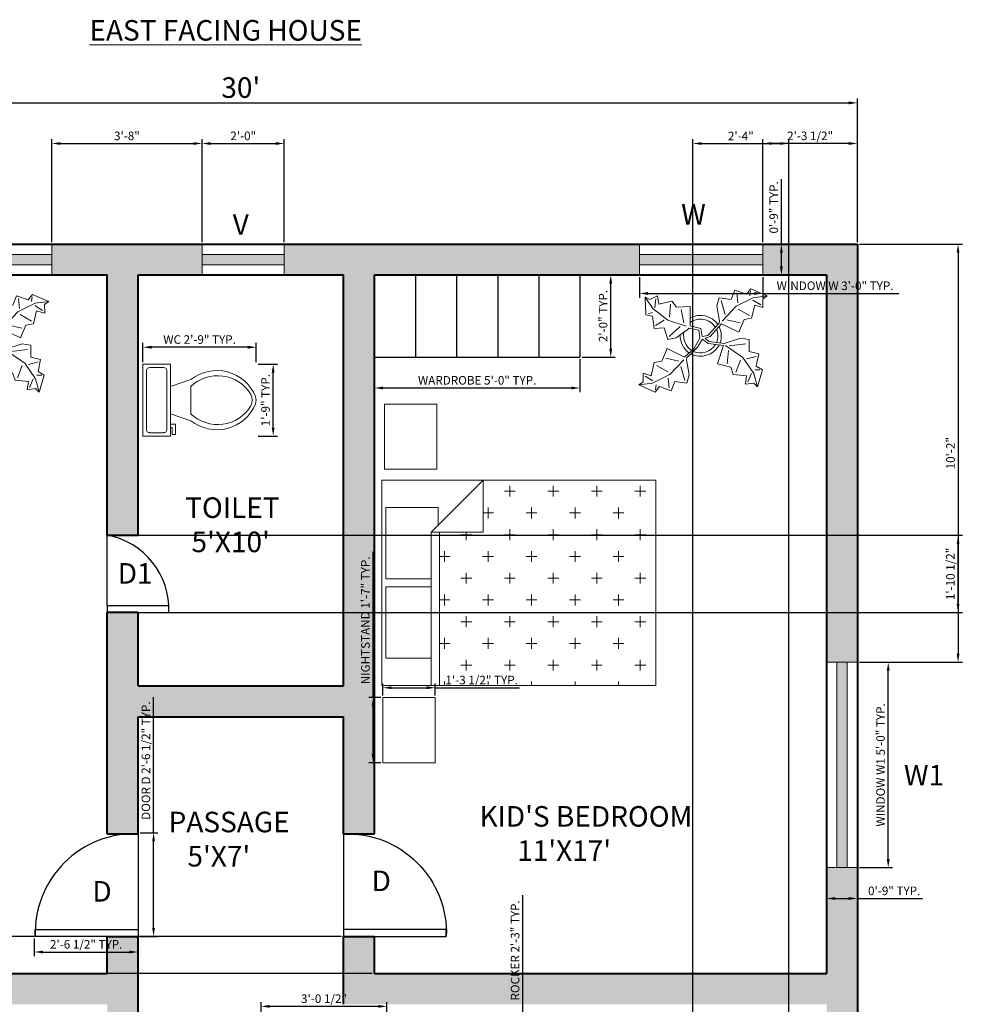
# Model space of a CAD drawing. Units: inches. Extents: x 4432 to 4859, y 8121 to 8698.
# Tile 4 of 4: x 4583 to 4859, y 8410 to 8698. Entities that reach past the tile are written whole.
import ezdxf

# ---------------------------------------------------------------- set-up
doc = ezdxf.new("R2010")
doc.units = ezdxf.units.IN
for name, color, linetype, lineweight in [('A-ANNO-DIMS', 2, 'Continuous', 18), ('A-ANNO-TEXT', 7, 'Continuous', 18), ('A-AREA-IDEN', 4, 'Continuous', 18), ('A-DOOR', 3, 'Continuous', 25), ('A-FLOR-CASE', 8, 'Continuous', 25), ('A-FLOR-FIXT', 9, 'Continuous', 18), ('A-FURN', 8, 'Continuous', 18), ('A-FURN-PATT', 8, 'Continuous', 13), ('A-FURN-PLNT', 94, 'Continuous', 13), ('A-GLAZ', 4, 'Continuous', 20), ('A-GLAZ-PATT', 4, 'Continuous', 13), ('A-WALL', 7, 'Continuous', 40)]:
    doc.layers.add(name, color=color, linetype=linetype, lineweight=lineweight)
doc.layers.add('A-WALL-PATT', color=219, linetype='Continuous', lineweight=13, true_color=0x642165)
doc.styles.get("Standard").update_dxf_attribs({"font": 'arial.ttf'})
doc.dimstyles.new('ISO-25', dxfattribs={"dimtxt": 2.5, "dimasz": 2.5, "dimexe": 1.25, "dimexo": 0.625, "dimtad": 1, "dimlunit": 3, "dimtxsty": 'Standard', "dimcen": 2.5, "dimadec": 0, "dimazin": 0, "dimtfac": 1, "dimtmove": 0, "dimatfit": 3, "dimfxl": 1, "dimarcsym": 0})

# ---------------------------------------------------------------- blocks, each defined once
blk = doc.blocks.new('Bed - Queen')
for p, q in [((0, -80.00003), (0, 0)), ((0, 0), (59.99999, 0)), ((59.99999, 0), (59.99999, -80.00003)), ((7.99999, -1.2), (28.79998, -1.2)), ((7.99999, -14.4), (7.99999, -1.2)), ((28.79998, -1.2), (28.79998, -14.4)), ((31.19999, -1.2), (51.99999, -1.2)), ((31.19999, -14.4), (31.19999, -1.2)), ((51.99999, -1.2), (51.99999, -16.4)), ((0, -14.4), (44.8, -14.4)), ((44.8, -16.8), (0, -16.8)), ((59.99999, -29.6), (44.8, -14.4)), ((44.8, -14.4), (44.8, -29.6)), ((51.99999, -16.4), (46.79936, -16.4)), ((44.8, -29.6), (59.99999, -29.6)), ((59.99999, -80.00003), (0, -80.00003))]:
    blk.add_line(p, q)
blk = doc.blocks.new('Plant - Rubber or Philodendron')
for p, q in [((-14.8639, 10.7964), (-12.6195, 11.8975)), ((-12.6195, 11.8975), (-12.1909, 9.4345)), ((8.8871, 10.7908), (9.9809, 13.4933)), ((9.9809, 13.4933), (13.3837, 12.301)), ((10.5828, 12.6946), (10.8893, 9.7953)), ((13.3837, 12.301), (14.68, 13.9039)), ((14.5816, 13.2037), (14.3848, 11.8033)), ((14.68, 13.9039), (19.3848, 11.8146)), ((19.3848, 11.8146), (15.3859, 11.3055)), ((19.3848, 11.8146), (18.1868, 10.9119)), ((-16.2005, 11.4774), (-13.9899, 8.1064)), ((-16.2005, 11.4774), (-14.8639, 10.7964)), ((-16.0159, 6.3329), (-16.2005, 11.4774)), ((-13.3174, 8.325), (-13.0735, 11.0065)), ((-12.1909, 9.4345), (-8.3829, 10.3)), ((-8.8369, 9.409), (-9.0894, 5.6095)), ((-8.3829, 10.3), (-7.0549, 8.501)), ((-7.0549, 8.501), (-3.0284, 8.6941)), ((-3.0284, 8.6941), (-3.0709, 3.1041)), ((4.6914, 8.8812), (5.3859, 11.2828)), ((4.6914, 8.8812), (5.5014, 4.4831)), ((5.3859, 11.2828), (8.8871, 10.7908)), ((5.9878, 10.4842), (7.1971, 6.3869)), ((10.3916, 8.7942), (6.2847, 4.4028)), ((15.3859, 11.3055), (10.3916, 8.7942)), ((15.7909, 9.1065), (14.8995, 5.3044)), ((15.2875, 10.6053), (17.5907, 9.2105)), ((18.1925, 8.4119), (15.7909, 9.1065)), ((18.1868, 10.9119), (18.1925, 8.4119)), ((-14.0069, 5.8704), (-16.0159, 6.3329)), ((-15.3434, 6.5514), (-13.9984, 6.9884)), ((-13.5868, 2.2894), (-14.0069, 5.8704)), ((-13.9899, 8.1064), (-9.5434, 4.7185)), ((-4.8529, 4.012), (-5.7184, 7.82)), ((14.2977, 6.1031), (10.9934, 7.9956)), ((-13.1329, 3.1804), (-10.6614, 4.727)), ((-9.5434, 4.7185), (-4.1917, 2.9888)), ((-9.1318, 0.0195), (-5.9793, 2.9025)), ((-3.0709, 3.1041), (0.0797, 2.3163)), ((2.1141, 0.2298), (5.4346, 3.9146)), ((6.1032, 3.6844), (2.8262, -0.031)), ((5.4346, 3.9146), (5.5014, 4.4831)), ((11.1089, 1.1958), (6.1032, 3.6844)), ((7.7005, 4.8881), (11.5025, 3.9967)), ((12.7005, 4.8994), (11.1089, 1.1958)), ((14.8995, 5.3044), (12.7005, 4.8994)), ((-10.6784, 2.491), (-13.5868, 2.2894)), ((-9.5858, -0.8715), (-10.6784, 2.491)), ((-7.1228, -0.443), (-3.5248, 2.2131)), ((-3.5248, 2.2131), (-3.3011, 2.4355)), ((-3.3011, 2.4355), (-0.5306, 1.7947)), ((-0.5306, 1.7947), (-0.2255, -0.5527)), ((-0.5306, 1.7947), (-0.5306, 1.7947)), ((0.0797, 2.3163), (0.4866, -0.031)), ((0.4866, -0.031), (2.1141, 0.2298)), ((-7.1228, -0.443), (-9.5858, -0.8715)), ((-2.019, -3.6148), (-0.2255, -0.5527)), ((-0.9375, -3.1608), (0.5883, -0.8135)), ((0.5883, -0.8135), (2.2447, -2.0916)), ((2.8262, -0.031), (1.3003, -0.5527)), ((1.3003, -0.5527), (2.4193, -1.4655)), ((2.2447, -2.0916), (6.7108, -2.6626)), ((2.4193, -1.4655), (6.895, -2.1175)), ((4.943, -7.9659), (6.7108, -2.6626)), ((11.6605, -0.5413), (6.895, -2.1175)), ((12.3677, -6.1981), (7.219, -2.6772)), ((8.3544, -2.7453), (13.1973, -2.1704)), ((11.6605, -0.5413), (14.1354, -0.8948)), ((14.1354, -0.8948), (14.1354, -4.4304)), ((-11.3237, -7.2629), (-9.7321, -3.5593)), ((-9.7321, -3.5593), (-4.7264, -6.0479)), ((-2.019, -3.6148), (-4.7264, -6.0479)), ((-4.0579, -6.2781), (-0.9375, -3.1608)), ((8.125, -4.0768), (7.7715, -7.9659)), ((14.1354, -4.4304), (16.9638, -5.1375)), ((16.9638, -5.1375), (16.2567, -8.673)), ((-14.4141, -11.4699), (-13.5228, -7.6679)), ((-13.5228, -7.6679), (-11.3237, -7.2629)), ((-12.921, -8.4665), (-9.6166, -10.359)), ((-6.3237, -7.2516), (-10.1257, -6.3602)), ((-9.0148, -11.1577), (-4.9047, -6.8122)), ((-4.1246, -6.8466), (-4.0579, -6.2781)), ((-3.3146, -11.2447), (-4.1246, -6.8466)), ((8.8321, -9.0266), (4.943, -7.9659)), ((10.2463, -10.4408), (11.6605, -6.9053)), ((15.5496, -10.7943), (12.3677, -6.1981)), ((16.2567, -5.8446), (13.4283, -6.5517)), ((-16.8157, -10.7754), (-14.4141, -11.4699)), ((-16.8101, -13.2754), (-16.8157, -10.7754)), ((-14.0091, -13.669), (-9.0148, -11.1577)), ((-4.611, -12.8477), (-5.8203, -8.7504)), ((-3.3146, -11.2447), (-4.0092, -13.6463)), ((9.5392, -11.1479), (8.8321, -9.0266)), ((13.4283, -11.5015), (9.5392, -11.1479)), ((13.0748, -13.9763), (13.4283, -11.5015)), ((14.8425, -10.7943), (13.7819, -13.2692)), ((16.6103, -14.6834), (15.5496, -10.7943)), ((17.3174, -9.7337), (15.9032, -9.7337)), ((16.2567, -8.673), (18.0245, -9.7337)), ((18.0245, -9.7337), (16.6103, -14.6834)), ((-18.008, -14.1781), (-16.8101, -13.2754)), ((-18.008, -14.1781), (-14.0091, -13.669)), ((-13.3032, -16.2674), (-18.008, -14.1781)), ((-13.9107, -12.9688), (-16.2139, -11.574)), ((-13.2048, -15.5672), (-13.008, -14.1668)), ((-9.206, -15.0581), (-9.5126, -12.1588)), ((-7.5103, -13.1543), (-8.6042, -15.8568)), ((-4.0092, -13.6463), (-7.5103, -13.1543)), ((15.5496, -13.6228), (13.0748, -13.9763)), ((16.6103, -14.6834), (15.5496, -13.6228)), ((-12.0069, -14.6645), (-13.3032, -16.2674)), ((-8.6042, -15.8568), (-12.0069, -14.6645))]:
    blk.add_line(p, q)
for centre, radius, start, end in [((0, 0), 6.1275, 34.37569, 120.1028), ((-0.0601, -0.2075), 5.2461, 33.82192, 124.9414), ((0.0308, 0.1664), 6, 178.6147, 235.1169), ((0.0308, 0.1664), 5, 168.1647, 238.6725), ((-0.2664, 0.1682), 5.2775, 338.4094, 20.03007), ((-0.098, 0.1364), 6.1288, 341.2017, 26.09184), ((-0.0234, 0.3825), 6.1492, 242.5812, 331.2714), ((-0.1102, 0.4886), 5.2883, 247.3711, 327.472)]:
    blk.add_arc(centre, radius, start, end)
blk = doc.blocks.new('Toilet - top')
for p, q in [((9.5, -6), (9.5, -2)), ((-10, -8.5), (-8, -8.5)), ((-10, -9.5), (-10, -8.5)), ((-8, -8.5), (-8, -8)), ((-7, -8), (-7, -9.5)), ((-4, -8), (-6, -14)), ((4, -8), (6, -14)), ((-7, -9.5), (-10, -9.5)), ((4, -14), (-4, -14))]:
    blk.add_line(p, q)
blk.add_lwpolyline([(10.5, -8), (10.5, 0), (-10.5, 0), (-10.5, -8)], close=True)
for points in [[(-9.5, -2), (-9.5, -6)], [(8.5, -1), (-8.5, -1)], [(-8.5, -7), (8.5, -7)]]:
    blk.add_lwpolyline(points)
for centre, radius, start, end in [((-8.62, -1.88), 0.884, 81.8699, 188.1301), ((8.62, -1.88), 0.884, 351.8699, 98.1301), ((-8.62, -6.12), 0.884, 171.8699, 278.1301), ((8.62, -6.12), 0.884, 261.8699, 8.1301), ((3.52, -21.58), 12.17, 141.4691, 247.9714), ((4.2, -21.82), 11.33, 136.3677, 238.9468), ((-3.52, -21.58), 12.17, 292.0284, 38.5307), ((-4.2, -21.82), 11.33, 301.053, 43.6321), ((0, -27.88), 4, 245.7318, 294.2682), ((0, -29), 4, 254.8605, 285.1395)]:
    blk.add_arc(centre, radius, start, end)
blk = doc.blocks.new('*D14')
at = {"layer": 'A-ANNO-DIMS', "color": 0, "lineweight": -2, "transparency": 16777216}
for p, q in [((4467.47, 8632.58), (4467.47, 8674.47)), ((4469.97, 8673.22), (4824.97, 8673.22)), ((4827.47, 8632.58), (4827.47, 8674.47))]:
    blk.add_line(p, q, dxfattribs=at)
at = {"layer": 'A-ANNO-DIMS', "color": 0, "transparency": 16777216}
for points in [[(4469.97, 8673.64), (4469.97, 8672.8), (4467.47, 8673.22)], [(4824.97, 8673.64), (4824.97, 8672.8), (4827.47, 8673.22)]]:
    blk.add_solid(points, dxfattribs=at)
at = {"layer": 'Defpoints', "color": 0, "transparency": 16777216}
for p in [(4827.47, 8673.22), (4467.47, 8631.96), (4827.47, 8631.96)]:
    blk.add_point(p, dxfattribs=at)
at = {"layer": 'A-ANNO-DIMS', "color": 0, "transparency": 16777216, "insert": (4647.47, 8676.91), "char_height": 6, "attachment_point": 5}
blk.add_mtext("30'", dxfattribs=at)
blk = doc.blocks.new('WIN-36IN')
for p, q in [((0, 0), (0, 9)), ((0, 9), (36, 9)), ((36, 9), (36, 0)), ((0, 6), (36, 6)), ((0, 3), (36, 3)), ((36, 0), (0, 0))]:
    blk.add_line(p, q)
blk = doc.blocks.new('WIN-60IN')
for p, q in [((0, 60), (9, 60)), ((0, 60), (0, 0)), ((3, 60), (3, 0)), ((6, 60), (6, 0)), ((9, 0), (9, 60)), ((0, 0), (9, 0)), ((0, 0), (9, 0))]:
    blk.add_line(p, q)
blk = doc.blocks.new('DOOR-SWING-30IN')
for p, q in [((0, 30), (0, 0)), ((-30, 0), (-30, 2)), ((-30, 2), (0, 2)), ((0, 0), (-30, 0))]:
    blk.add_line(p, q)
blk.add_arc((-1, 1), 29.02, 88.0251, 181.9749)
blk = doc.blocks.new('WARDROBE-5BAY-60IN')
for p, q in [((12, 24), (12, 0)), ((24, 24), (24, 0)), ((36, 24), (36, 0)), ((48, 24), (48, 0)), ((60, 24), (60, 0)), ((0, 0), (60, 0))]:
    blk.add_line(p, q)
blk = doc.blocks.new('NIGHTSTAND-RECT')
blk.add_lwpolyline([(0, 19.04), (15.29, 19.04), (15.29, 0), (0, 0)], close=True)
blk = doc.blocks.new('*D23')
at = {"layer": 'A-ANNO-DIMS', "color": 0, "lineweight": -2, "transparency": 16777216}
for p, q in [((4763.88, 8622.33), (4763.88, 8616.31)), ((4799.88, 8622.33), (4799.88, 8616.31)), ((4766.38, 8617.56), (4797.38, 8617.56)), ((4799.88, 8617.56), (4839.53, 8617.56))]:
    blk.add_line(p, q, dxfattribs=at)
at = {"layer": 'A-ANNO-DIMS', "color": 0, "transparency": 16777216}
for points in [[(4766.38, 8617.97), (4766.38, 8617.14), (4763.88, 8617.56)], [(4797.38, 8617.97), (4797.38, 8617.14), (4799.88, 8617.56)]]:
    blk.add_solid(points, dxfattribs=at)
at = {"layer": 'Defpoints', "color": 0, "transparency": 16777216}
for p in [(4763.88, 8622.96), (4799.88, 8622.96), (4799.88, 8617.56)]:
    blk.add_point(p, dxfattribs=at)
at = {"layer": 'A-ANNO-DIMS', "color": 0, "transparency": 16777216, "insert": (4820.95, 8619.48), "char_height": 2.5, "attachment_point": 5}
blk.add_mtext('WINDOW W 3\'-0" TYP.', dxfattribs=at)
blk = doc.blocks.new('*D24')
at = {"layer": 'A-ANNO-DIMS', "color": 0, "lineweight": -2, "transparency": 16777216}
for p, q in [((4805.28, 8631.96), (4805.28, 8650.95)), ((4800.5, 8631.96), (4806.53, 8631.96)), ((4805.28, 8625.46), (4805.28, 8629.46)), ((4800.5, 8622.96), (4806.53, 8622.96))]:
    blk.add_line(p, q, dxfattribs=at)
at = {"layer": 'A-ANNO-DIMS', "color": 0, "transparency": 16777216}
for points in [[(4804.86, 8629.46), (4805.69, 8629.46), (4805.28, 8631.96)], [(4804.86, 8625.46), (4805.69, 8625.46), (4805.28, 8622.96)]]:
    blk.add_solid(points, dxfattribs=at)
at = {"layer": 'Defpoints', "color": 0, "transparency": 16777216}
for p in [(4799.88, 8631.96), (4805.28, 8631.96), (4799.88, 8622.96)]:
    blk.add_point(p, dxfattribs=at)
at = {"layer": 'A-ANNO-DIMS', "color": 0, "transparency": 16777216, "insert": (4803.38, 8642.7), "char_height": 2.5, "attachment_point": 5, "rotation": 90}
blk.add_mtext('0\'-9" TYP.', dxfattribs=at)
blk = doc.blocks.new('*D25')
at = {"layer": 'A-ANNO-DIMS', "color": 0, "lineweight": -2, "transparency": 16777216}
for p, q in [((4828.09, 8509.87), (4837.72, 8509.87)), ((4836.47, 8452.37), (4836.47, 8507.37)), ((4828.09, 8449.87), (4837.72, 8449.87))]:
    blk.add_line(p, q, dxfattribs=at)
at = {"layer": 'A-ANNO-DIMS', "color": 0, "transparency": 16777216}
for points in [[(4836.05, 8507.37), (4836.88, 8507.37), (4836.47, 8509.87)], [(4836.05, 8452.37), (4836.88, 8452.37), (4836.47, 8449.87)]]:
    blk.add_solid(points, dxfattribs=at)
at = {"layer": 'Defpoints', "color": 0, "transparency": 16777216}
for p in [(4827.47, 8509.87), (4836.47, 8509.87), (4827.47, 8449.87)]:
    blk.add_point(p, dxfattribs=at)
at = {"layer": 'A-ANNO-DIMS', "color": 0, "transparency": 16777216, "insert": (4834.55, 8479.87), "char_height": 2.5, "attachment_point": 5, "rotation": 90}
blk.add_mtext('WINDOW W1 5\'-0" TYP.', dxfattribs=at)
blk = doc.blocks.new('*D26')
at = {"layer": 'A-ANNO-DIMS', "color": 0, "lineweight": -2, "transparency": 16777216}
for p, q in [((4818.47, 8449.25), (4818.47, 8439.62)), ((4827.47, 8449.25), (4827.47, 8439.62)), ((4820.97, 8440.87), (4824.97, 8440.87)), ((4827.47, 8440.87), (4846.46, 8440.87))]:
    blk.add_line(p, q, dxfattribs=at)
at = {"layer": 'A-ANNO-DIMS', "color": 0, "transparency": 16777216}
for points in [[(4820.97, 8441.29), (4820.97, 8440.45), (4818.47, 8440.87)], [(4824.97, 8441.29), (4824.97, 8440.45), (4827.47, 8440.87)]]:
    blk.add_solid(points, dxfattribs=at)
at = {"layer": 'Defpoints', "color": 0, "transparency": 16777216}
for p in [(4818.47, 8449.87), (4827.47, 8449.87), (4827.47, 8440.87)]:
    blk.add_point(p, dxfattribs=at)
at = {"layer": 'A-ANNO-DIMS', "color": 0, "transparency": 16777216, "insert": (4838.21, 8442.77), "char_height": 2.5, "attachment_point": 5}
blk.add_mtext('0\'-9" TYP.', dxfattribs=at)
blk = doc.blocks.new('*D29')
at = {"layer": 'A-ANNO-DIMS', "color": 0, "lineweight": -2, "transparency": 16777216}
for p, q in [((4686.1, 8499.56), (4686.1, 8542.1)), ((4688.33, 8499.56), (4684.85, 8499.56)), ((4686.1, 8483.02), (4686.1, 8497.06)), ((4688.33, 8480.52), (4684.85, 8480.52))]:
    blk.add_line(p, q, dxfattribs=at)
at = {"layer": 'A-ANNO-DIMS', "color": 0, "transparency": 16777216}
for points in [[(4685.68, 8497.06), (4686.51, 8497.06), (4686.1, 8499.56)], [(4685.68, 8483.02), (4686.51, 8483.02), (4686.1, 8480.52)]]:
    blk.add_solid(points, dxfattribs=at)
at = {"layer": 'Defpoints', "color": 0, "transparency": 16777216}
for p in [(4686.1, 8499.56), (4688.95, 8499.56), (4688.95, 8480.52)]:
    blk.add_point(p, dxfattribs=at)
at = {"layer": 'A-ANNO-DIMS', "color": 0, "transparency": 16777216, "insert": (4684.18, 8522.08), "char_height": 2.5, "attachment_point": 5, "rotation": 90}
blk.add_mtext('NIGHTSTAND 1\'-7" TYP.', dxfattribs=at)
blk = doc.blocks.new('*D30')
at = {"layer": 'A-ANNO-DIMS', "color": 0, "lineweight": -2, "transparency": 16777216}
for p, q in [((4688.95, 8500.18), (4688.95, 8503.66)), ((4704.24, 8500.18), (4704.24, 8503.66)), ((4691.45, 8502.41), (4701.74, 8502.41)), ((4704.24, 8502.41), (4728.82, 8502.41))]:
    blk.add_line(p, q, dxfattribs=at)
at = {"layer": 'A-ANNO-DIMS', "color": 0, "transparency": 16777216}
for points in [[(4691.45, 8502.83), (4691.45, 8502), (4688.95, 8502.41)], [(4701.74, 8502.83), (4701.74, 8502), (4704.24, 8502.41)]]:
    blk.add_solid(points, dxfattribs=at)
at = {"layer": 'Defpoints', "color": 0, "transparency": 16777216}
for p in [(4704.24, 8502.41), (4688.95, 8499.56), (4704.24, 8499.56)]:
    blk.add_point(p, dxfattribs=at)
at = {"layer": 'A-ANNO-DIMS', "color": 0, "transparency": 16777216, "insert": (4717.78, 8504.33), "char_height": 2.5, "attachment_point": 5}
blk.add_mtext('1\'-3 1/2" TYP.', dxfattribs=at)
blk = doc.blocks.new('*D31')
at = {"layer": 'A-ANNO-DIMS', "color": 0, "lineweight": -2, "transparency": 16777216}
for p, q in [((4622.01, 8460.05), (4622.01, 8499.68)), ((4618.09, 8460.05), (4623.26, 8460.05)), ((4622.01, 8432.28), (4622.01, 8457.55)), ((4618.09, 8429.78), (4623.26, 8429.78))]:
    blk.add_line(p, q, dxfattribs=at)
at = {"layer": 'A-ANNO-DIMS', "color": 0, "transparency": 16777216}
for points in [[(4621.59, 8457.55), (4622.43, 8457.55), (4622.01, 8460.05)], [(4621.59, 8432.28), (4622.43, 8432.28), (4622.01, 8429.78)]]:
    blk.add_solid(points, dxfattribs=at)
at = {"layer": 'Defpoints', "color": 0, "transparency": 16777216}
for p in [(4617.47, 8460.05), (4622.01, 8460.05), (4617.47, 8429.78)]:
    blk.add_point(p, dxfattribs=at)
at = {"layer": 'A-ANNO-DIMS', "color": 0, "transparency": 16777216, "insert": (4620.09, 8481.12), "char_height": 2.5, "attachment_point": 5, "rotation": 90}
blk.add_mtext('DOOR D 2\'-6 1/2" TYP.', dxfattribs=at)
blk = doc.blocks.new('*D32')
at = {"layer": 'A-ANNO-DIMS', "color": 0, "lineweight": -2, "transparency": 16777216}
for p, q in [((4587.19, 8429.15), (4587.19, 8423.98)), ((4617.47, 8429.15), (4617.47, 8423.98)), ((4589.69, 8425.23), (4614.97, 8425.23))]:
    blk.add_line(p, q, dxfattribs=at)
at = {"layer": 'A-ANNO-DIMS', "color": 0, "transparency": 16777216}
for points in [[(4589.69, 8425.65), (4589.69, 8424.82), (4587.19, 8425.23)], [(4614.97, 8425.65), (4614.97, 8424.82), (4617.47, 8425.23)]]:
    blk.add_solid(points, dxfattribs=at)
at = {"layer": 'Defpoints', "color": 0, "transparency": 16777216}
for p in [(4587.19, 8429.78), (4617.47, 8429.78), (4617.47, 8425.23)]:
    blk.add_point(p, dxfattribs=at)
at = {"layer": 'A-ANNO-DIMS', "color": 0, "transparency": 16777216, "insert": (4602.33, 8427.15), "char_height": 2.5, "attachment_point": 5}
blk.add_mtext('2\'-6 1/2" TYP.', dxfattribs=at)
blk = doc.blocks.new('*D33')
at = {"layer": 'A-ANNO-DIMS', "color": 0, "lineweight": -2, "transparency": 16777216}
for p, q in [((4729.79, 8407.06), (4729.79, 8441.83)), ((4726.37, 8407.06), (4731.04, 8407.06)), ((4729.79, 8382.56), (4729.79, 8404.56)), ((4726.37, 8380.06), (4731.04, 8380.06))]:
    blk.add_line(p, q, dxfattribs=at)
at = {"layer": 'A-ANNO-DIMS', "color": 0, "transparency": 16777216}
for points in [[(4729.38, 8404.56), (4730.21, 8404.56), (4729.79, 8407.06)], [(4729.38, 8382.56), (4730.21, 8382.56), (4729.79, 8380.06)]]:
    blk.add_solid(points, dxfattribs=at)
at = {"layer": 'Defpoints', "color": 0, "transparency": 16777216}
for p in [(4725.74, 8407.06), (4729.79, 8407.06), (4725.74, 8380.06)]:
    blk.add_point(p, dxfattribs=at)
at = {"layer": 'A-ANNO-DIMS', "color": 0, "transparency": 16777216, "insert": (4727.87, 8425.7), "char_height": 2.5, "attachment_point": 5, "rotation": 90}
blk.add_mtext('ROCKER 2\'-3" TYP.', dxfattribs=at)
blk = doc.blocks.new('*D37')
at = {"layer": 'A-ANNO-DIMS', "color": 0, "lineweight": -2, "transparency": 16777216}
for p, q in [((4618.91, 8597.53), (4618.91, 8603.11)), ((4649.46, 8601.86), (4621.41, 8601.86)), ((4651.96, 8597.53), (4651.96, 8603.11))]:
    blk.add_line(p, q, dxfattribs=at)
at = {"layer": 'A-ANNO-DIMS', "color": 0, "transparency": 16777216}
for points in [[(4621.41, 8602.28), (4621.41, 8601.44), (4618.91, 8601.86)], [(4649.46, 8602.28), (4649.46, 8601.44), (4651.96, 8601.86)]]:
    blk.add_solid(points, dxfattribs=at)
at = {"layer": 'Defpoints', "color": 0, "transparency": 16777216}
for p in [(4618.91, 8601.86), (4618.91, 8596.9), (4651.96, 8596.9)]:
    blk.add_point(p, dxfattribs=at)
at = {"layer": 'A-ANNO-DIMS', "color": 0, "transparency": 16777216, "insert": (4635.44, 8603.78), "char_height": 2.5, "attachment_point": 5}
blk.add_mtext('WC 2\'-9" TYP.', dxfattribs=at)
blk = doc.blocks.new('*D38')
at = {"layer": 'A-ANNO-DIMS', "color": 0, "lineweight": -2, "transparency": 16777216}
for p, q in [((4652.58, 8596.9), (4658.17, 8596.9)), ((4656.92, 8578.4), (4656.92, 8594.4)), ((4652.58, 8575.9), (4658.17, 8575.9))]:
    blk.add_line(p, q, dxfattribs=at)
at = {"layer": 'A-ANNO-DIMS', "color": 0, "transparency": 16777216}
for points in [[(4656.5, 8594.4), (4657.33, 8594.4), (4656.92, 8596.9)], [(4656.5, 8578.4), (4657.33, 8578.4), (4656.92, 8575.9)]]:
    blk.add_solid(points, dxfattribs=at)
at = {"layer": 'Defpoints', "color": 0, "transparency": 16777216}
for p in [(4651.96, 8596.9), (4656.92, 8596.9), (4651.96, 8575.9)]:
    blk.add_point(p, dxfattribs=at)
at = {"layer": 'A-ANNO-DIMS', "color": 0, "transparency": 16777216, "insert": (4655.02, 8586.4), "char_height": 2.5, "attachment_point": 5, "rotation": 90}
blk.add_mtext('1\'-9" TYP.', dxfattribs=at)
blk = doc.blocks.new('*D43')
at = {"layer": 'A-ANNO-DIMS', "color": 0, "lineweight": -2, "transparency": 16777216}
for p, q in [((4686.47, 8598.33), (4686.47, 8588.71)), ((4746.47, 8598.33), (4746.47, 8588.71)), ((4688.97, 8589.96), (4743.97, 8589.96))]:
    blk.add_line(p, q, dxfattribs=at)
at = {"layer": 'A-ANNO-DIMS', "color": 0, "transparency": 16777216}
for points in [[(4688.97, 8590.37), (4688.97, 8589.54), (4686.47, 8589.96)], [(4743.97, 8590.37), (4743.97, 8589.54), (4746.47, 8589.96)]]:
    blk.add_solid(points, dxfattribs=at)
at = {"layer": 'Defpoints', "color": 0, "transparency": 16777216}
for p in [(4686.47, 8598.96), (4746.47, 8598.96), (4746.47, 8589.96)]:
    blk.add_point(p, dxfattribs=at)
at = {"layer": 'A-ANNO-DIMS', "color": 0, "transparency": 16777216, "insert": (4716.47, 8591.87), "char_height": 2.5, "attachment_point": 5}
blk.add_mtext('WARDROBE 5\'-0" TYP.', dxfattribs=at)
blk = doc.blocks.new('*D44')
at = {"layer": 'A-ANNO-DIMS', "color": 0, "lineweight": -2, "transparency": 16777216}
for p, q in [((4747.09, 8622.96), (4756.72, 8622.96)), ((4755.47, 8601.46), (4755.47, 8620.46)), ((4747.09, 8598.96), (4756.72, 8598.96))]:
    blk.add_line(p, q, dxfattribs=at)
at = {"layer": 'A-ANNO-DIMS', "color": 0, "transparency": 16777216}
for points in [[(4755.05, 8620.46), (4755.88, 8620.46), (4755.47, 8622.96)], [(4755.05, 8601.46), (4755.88, 8601.46), (4755.47, 8598.96)]]:
    blk.add_solid(points, dxfattribs=at)
at = {"layer": 'Defpoints', "color": 0, "transparency": 16777216}
for p in [(4746.47, 8622.96), (4755.47, 8622.96), (4746.47, 8598.96)]:
    blk.add_point(p, dxfattribs=at)
at = {"layer": 'A-ANNO-DIMS', "color": 0, "transparency": 16777216, "insert": (4753.57, 8610.96), "char_height": 2.5, "attachment_point": 5, "rotation": 90}
blk.add_mtext('2\'-0" TYP.', dxfattribs=at)
blk = doc.blocks.new('*D50')
at = {"layer": 'A-ANNO-DIMS', "color": 0, "lineweight": -2, "transparency": 16777216}
for p, q in [((4653.44, 8397.38), (4653.44, 8410.61)), ((4687.61, 8409.36), (4655.94, 8409.36)), ((4690.11, 8397.38), (4690.11, 8410.61))]:
    blk.add_line(p, q, dxfattribs=at)
at = {"layer": 'A-ANNO-DIMS', "color": 0, "transparency": 16777216}
for points in [[(4655.94, 8409.77), (4655.94, 8408.94), (4653.44, 8409.36)], [(4687.61, 8409.77), (4687.61, 8408.94), (4690.11, 8409.36)]]:
    blk.add_solid(points, dxfattribs=at)
at = {"layer": 'Defpoints', "color": 0, "transparency": 16777216}
for p in [(4653.44, 8409.36), (4653.44, 8396.76), (4690.11, 8396.76)]:
    blk.add_point(p, dxfattribs=at)
at = {"layer": 'A-ANNO-DIMS', "color": 0, "transparency": 16777216, "insert": (4671.77, 8411.28), "char_height": 2.5, "attachment_point": 5}
blk.add_mtext('3\'-0 1/2"', dxfattribs=at)
blk = doc.blocks.new('*D52')
at = {"layer": 'A-ANNO-DIMS', "color": 0, "lineweight": -2, "transparency": 16777216}
for p, q in [((4592.31, 8632.58), (4592.31, 8662.61)), ((4594.81, 8661.36), (4633.68, 8661.36)), ((4636.18, 8632.58), (4636.18, 8662.61))]:
    blk.add_line(p, q, dxfattribs=at)
at = {"layer": 'A-ANNO-DIMS', "color": 0, "transparency": 16777216}
for points in [[(4594.81, 8661.77), (4594.81, 8660.94), (4592.31, 8661.36)], [(4633.68, 8661.77), (4633.68, 8660.94), (4636.18, 8661.36)]]:
    blk.add_solid(points, dxfattribs=at)
at = {"layer": 'Defpoints', "color": 0, "transparency": 16777216}
for p in [(4636.18, 8661.36), (4592.31, 8631.96), (4636.18, 8631.96)]:
    blk.add_point(p, dxfattribs=at)
at = {"layer": 'A-ANNO-DIMS', "color": 0, "transparency": 16777216, "insert": (4614.24, 8663.26), "char_height": 2.5, "attachment_point": 5}
blk.add_mtext('3\'-8"', dxfattribs=at)
blk = doc.blocks.new('*D53')
at = {"layer": 'A-ANNO-DIMS', "color": 0, "lineweight": -2, "transparency": 16777216}
for p, q in [((4799.88, 8632.58), (4799.88, 8662.61)), ((4824.97, 8661.36), (4802.38, 8661.36)), ((4827.47, 8632.58), (4827.47, 8662.61))]:
    blk.add_line(p, q, dxfattribs=at)
at = {"layer": 'A-ANNO-DIMS', "color": 0, "transparency": 16777216}
for points in [[(4802.38, 8661.77), (4802.38, 8660.94), (4799.88, 8661.36)], [(4824.97, 8661.77), (4824.97, 8660.94), (4827.47, 8661.36)]]:
    blk.add_solid(points, dxfattribs=at)
at = {"layer": 'Defpoints', "color": 0, "transparency": 16777216}
for p in [(4799.88, 8661.36), (4799.88, 8631.96), (4827.47, 8631.96)]:
    blk.add_point(p, dxfattribs=at)
at = {"layer": 'A-ANNO-DIMS', "color": 0, "transparency": 16777216, "insert": (4813.67, 8663.27), "char_height": 2.5, "attachment_point": 5}
blk.add_mtext('2\'-3 1/2"', dxfattribs=at)
blk = doc.blocks.new('*D54')
at = {"layer": 'A-ANNO-DIMS', "color": 0, "lineweight": -2, "transparency": 16777216}
for p, q in [((4636.18, 8632.58), (4636.18, 8662.61)), ((4638.68, 8661.36), (4657.68, 8661.36)), ((4660.18, 8632.58), (4660.18, 8662.61))]:
    blk.add_line(p, q, dxfattribs=at)
at = {"layer": 'A-ANNO-DIMS', "color": 0, "transparency": 16777216}
for points in [[(4638.68, 8661.77), (4638.68, 8660.94), (4636.18, 8661.36)], [(4657.68, 8661.77), (4657.68, 8660.94), (4660.18, 8661.36)]]:
    blk.add_solid(points, dxfattribs=at)
at = {"layer": 'Defpoints', "color": 0, "transparency": 16777216}
for p in [(4660.18, 8661.36), (4636.18, 8631.96), (4660.18, 8631.96)]:
    blk.add_point(p, dxfattribs=at)
at = {"layer": 'A-ANNO-DIMS', "color": 0, "transparency": 16777216, "insert": (4648.18, 8663.26), "char_height": 2.5, "attachment_point": 5}
blk.add_mtext('2\'-0"', dxfattribs=at)
blk = doc.blocks.new('*D64')
at = {"layer": 'A-ANNO-DIMS', "color": 0, "lineweight": -2, "transparency": 16777216}
for p, q in [((4828.09, 8631.96), (4858.12, 8631.96)), ((4856.87, 8629.46), (4856.87, 8512.37)), ((4828.09, 8509.87), (4858.12, 8509.87))]:
    blk.add_line(p, q, dxfattribs=at)
at = {"layer": 'A-ANNO-DIMS', "color": 0, "transparency": 16777216}
for points in [[(4856.45, 8629.46), (4857.28, 8629.46), (4856.87, 8631.96)], [(4856.45, 8512.37), (4857.28, 8512.37), (4856.87, 8509.87)]]:
    blk.add_solid(points, dxfattribs=at)
at = {"layer": 'Defpoints', "color": 0, "transparency": 16777216}
for p in [(4827.47, 8631.96), (4827.47, 8509.87), (4856.87, 8509.87)]:
    blk.add_point(p, dxfattribs=at)
at = {"layer": 'A-ANNO-DIMS', "color": 0, "transparency": 16777216, "insert": (4854.97, 8570.91), "char_height": 2.5, "attachment_point": 5, "rotation": 90}
blk.add_mtext('10\'-2"', dxfattribs=at)
blk = doc.blocks.new('*D69')
at = {"layer": 'A-ANNO-DIMS', "color": 0, "lineweight": -2, "transparency": 16777216}
for p, q in [((4779.44, 8334.08), (4779.44, 8662.61)), ((4781.94, 8661.36), (4804.94, 8661.36)), ((4807.44, 8334.08), (4807.44, 8662.61))]:
    blk.add_line(p, q, dxfattribs=at)
at = {"layer": 'A-ANNO-DIMS', "color": 0, "transparency": 16777216}
for points in [[(4781.94, 8661.77), (4781.94, 8660.94), (4779.44, 8661.36)], [(4804.94, 8661.77), (4804.94, 8660.94), (4807.44, 8661.36)]]:
    blk.add_solid(points, dxfattribs=at)
at = {"layer": 'Defpoints', "color": 0, "transparency": 16777216}
for p in [(4807.44, 8661.36), (4779.44, 8333.46), (4807.44, 8333.46)]:
    blk.add_point(p, dxfattribs=at)
at = {"layer": 'A-ANNO-DIMS', "color": 0, "transparency": 16777216, "insert": (4793.44, 8663.24), "char_height": 2.5, "attachment_point": 5}
blk.add_mtext('2\'-4"', dxfattribs=at)
blk = doc.blocks.new('*D71')
at = {"layer": 'A-ANNO-DIMS', "color": 0, "lineweight": -2, "transparency": 16777216}
for p, q in [((4609.09, 8546.94), (4858.12, 8546.94)), ((4856.87, 8526.85), (4856.87, 8544.44)), ((4609.09, 8524.35), (4858.12, 8524.35))]:
    blk.add_line(p, q, dxfattribs=at)
at = {"layer": 'A-ANNO-DIMS', "color": 0, "transparency": 16777216}
for points in [[(4856.45, 8544.44), (4857.28, 8544.44), (4856.87, 8546.94)], [(4856.45, 8526.85), (4857.28, 8526.85), (4856.87, 8524.35)]]:
    blk.add_solid(points, dxfattribs=at)
at = {"layer": 'Defpoints', "color": 0, "transparency": 16777216}
for p in [(4608.47, 8546.94), (4856.87, 8546.94), (4608.47, 8524.35)]:
    blk.add_point(p, dxfattribs=at)
at = {"layer": 'A-ANNO-DIMS', "color": 0, "transparency": 16777216, "insert": (4854.95, 8535.65), "char_height": 2.5, "attachment_point": 5, "rotation": 90}
blk.add_mtext('1\'-10 1/2"', dxfattribs=at)
blk = doc.blocks.new('*D73')
at = {"layer": 'A-ANNO-DIMS', "color": 0, "lineweight": -2, "transparency": 16777216}
for p, q in [((4676.84, 8429.78), (4436.82, 8429.78)), ((4438.07, 8421.46), (4438.07, 8427.28)), ((4685.84, 8418.96), (4436.82, 8418.96))]:
    blk.add_line(p, q, dxfattribs=at)
at = {"layer": 'A-ANNO-DIMS', "color": 0, "transparency": 16777216}
for points in [[(4437.65, 8427.28), (4438.48, 8427.28), (4438.07, 8429.78)], [(4437.65, 8421.46), (4438.48, 8421.46), (4438.07, 8418.96)]]:
    blk.add_solid(points, dxfattribs=at)
at = {"layer": 'Defpoints', "color": 0, "transparency": 16777216}
for p in [(4438.07, 8429.78), (4677.47, 8429.78), (4686.47, 8418.96)]:
    blk.add_point(p, dxfattribs=at)
at = {"layer": 'A-ANNO-DIMS', "color": 0, "transparency": 16777216, "insert": (4436.17, 8424.37), "char_height": 2.5, "attachment_point": 5, "rotation": 90}
blk.add_mtext('0\'-11"', dxfattribs=at)

msp = doc.modelspace()

# ---------------------------------------------------------------- hatches: boundary and pattern name
at = {"layer": 'A-FURN-PATT'}
h = msp.add_hatch(dxfattribs=at)
h.set_pattern_fill('CROSS', color=256)
h.paths.add_polyline_path([(4558.735, 8563.044), (4508.335, 8563.044), (4508.335, 8547.844), (4495.535, 8547.844), (4495.535, 8503.044), (4558.735, 8503.044)])
h.paths.add_polyline_path([(4768.654, 8563.044), (4718.254, 8563.044), (4718.254, 8547.844), (4705.454, 8547.844), (4705.454, 8503.044), (4768.654, 8503.044)])
h.paths.add_polyline_path([(4699.088, 8354.439, 1), (4726.919, 8354.439, 1)])
at = {"layer": 'A-GLAZ-PATT'}
h = msp.add_hatch(color=256, dxfattribs=at)
h.dxf.hatch_style = 1
h.paths.add_polyline_path([(4592.313, 8628.956), (4556.313, 8628.956), (4556.313, 8625.956), (4592.313, 8625.956)])
h.paths.add_polyline_path([(4660.176, 8628.956), (4636.176, 8628.956), (4636.176, 8625.956), (4660.176, 8625.956)])
h.paths.add_polyline_path([(4799.877, 8628.956), (4763.877, 8628.956), (4763.877, 8625.956), (4799.877, 8625.956)])
h.paths.add_polyline_path([(4473.468, 8508.361), (4470.468, 8508.361), (4470.468, 8448.361), (4473.468, 8448.361)])
h.paths.add_polyline_path([(4473.468, 8398.047), (4470.468, 8398.047), (4470.468, 8377.047), (4473.468, 8377.047)])
h.paths.add_polyline_path([(4473.468, 8341.903), (4470.468, 8341.903), (4470.468, 8305.903), (4473.468, 8305.903)])
h.paths.add_polyline_path([(4577.354, 8253.956), (4529.354, 8253.956), (4529.354, 8250.956), (4577.354, 8250.956)])
h.paths.add_polyline_path([(4662.104, 8253.956), (4650.104, 8253.956), (4650.104, 8250.956), (4662.104, 8250.956)])
h.paths.add_polyline_path([(4722.104, 8253.956), (4710.104, 8253.956), (4710.104, 8250.956), (4722.104, 8250.956)])
h.paths.add_polyline_path([(4824.468, 8397.007), (4821.468, 8397.007), (4821.468, 8361.007), (4824.468, 8361.007)])
h.paths.add_polyline_path([(4824.468, 8509.871), (4821.468, 8509.871), (4821.468, 8449.871), (4824.468, 8449.871)])
at = {"layer": 'A-WALL-PATT'}
h = msp.add_hatch(color=256, dxfattribs=at)
h.dxf.hatch_style = 1
h.paths.add_polyline_path([(4556.313, 8631.956), (4467.468, 8631.956), (4467.468, 8508.361), (4476.468, 8508.361), (4476.468, 8622.956), (4556.313, 8622.956)])
h.paths.add_polyline_path([(4636.176, 8631.956), (4592.313, 8631.956), (4592.313, 8622.956), (4608.468, 8622.956), (4608.468, 8546.941), (4617.468, 8546.941), (4617.468, 8622.956), (4636.176, 8622.956)])
h.paths.add_polyline_path([(4763.877, 8631.956), (4660.176, 8631.956), (4660.176, 8622.956), (4677.468, 8622.956), (4677.468, 8502.956), (4617.468, 8502.956), (4617.468, 8524.355), (4608.468, 8524.355), (4608.468, 8459.776), (4615.468, 8459.776, -0.0172363), (4617.468, 8459.776), (4617.468, 8493.956), (4677.468, 8493.956), (4677.468, 8459.776, -0.0172363), (4679.468, 8459.776), (4686.468, 8459.776), (4686.468, 8622.956), (4763.877, 8622.956)])
h.paths.add_polyline_path([(4827.468, 8631.956), (4799.877, 8631.956), (4799.877, 8622.956), (4818.468, 8622.956), (4818.468, 8509.871), (4827.468, 8509.871)])
h.paths.add_polyline_path([(4617.468, 8429.776), (4608.468, 8429.776), (4608.468, 8418.956), (4476.468, 8418.956), (4476.468, 8448.361), (4467.468, 8448.361), (4467.468, 8398.047), (4476.468, 8398.047), (4476.468, 8409.956), (4608.468, 8409.956), (4608.468, 8397.41), (4612.05, 8397.41, -0.0497121), (4617.468, 8397.41)])
h.paths.add_polyline_path([(4827.468, 8449.871), (4818.468, 8449.871), (4818.468, 8418.956), (4686.468, 8418.956), (4686.468, 8429.776), (4677.468, 8429.776), (4677.468, 8409.956), (4818.468, 8409.956), (4818.468, 8397.007), (4827.468, 8397.007)])
h.paths.add_polyline_path([(4617.468, 8369.235), (4608.468, 8369.235), (4608.468, 8361.956), (4476.468, 8361.956), (4476.468, 8377.047), (4467.468, 8377.047), (4467.468, 8341.903), (4476.468, 8341.903), (4476.468, 8352.956), (4617.468, 8352.956)])
h.paths.add_polyline_path([(4529.354, 8256.956), (4476.468, 8256.956), (4476.468, 8305.903), (4467.468, 8305.903), (4467.468, 8151.956), (4650.104, 8151.956), (4650.104, 8157.956), (4471.968, 8157.956), (4471.968, 8169.956), (4599.396, 8169.956), (4599.396, 8174.456), (4476.468, 8174.456), (4476.468, 8247.956), (4529.354, 8247.956)])
h.paths.add_polyline_path([(4650.104, 8256.956), (4617.468, 8256.956), (4617.468, 8304.956), (4608.468, 8304.956), (4608.468, 8256.956), (4577.354, 8256.956), (4577.354, 8247.956), (4650.104, 8247.956)], flags=17)
h.paths.add_polyline_path([(4827.468, 8361.007), (4818.468, 8361.007), (4818.468, 8333.456), (4807.435, 8333.456, -0.0172363), (4807.435, 8331.456), (4807.435, 8328.956), (4818.468, 8328.956), (4818.468, 8256.956), (4770.468, 8256.956), (4770.468, 8328.956), (4777.435, 8328.956), (4777.435, 8333.456), (4765.968, 8333.456), (4765.968, 8256.956), (4722.104, 8256.956), (4722.104, 8247.956), (4821.468, 8247.956), (4821.468, 8157.956), (4765.968, 8157.956), (4765.968, 8151.956), (4827.468, 8151.956)])
h.paths.add_polyline_path([(4765.968, 8154.956), (4650.104, 8154.956), (4650.104, 8151.956), (4765.968, 8151.956)])

# ---------------------------------------------------------------- linework, layer by layer
at = {"layer": 'A-DOOR'}
for p, q in [((4608.468, 8526.355), (4608.468, 8546.941)), ((4626.468, 8526.355), (4608.468, 8526.355)), ((4608.468, 8526.355), (4608.468, 8524.355)), ((4626.468, 8524.355), (4626.468, 8526.355)), ((4608.468, 8524.355), (4626.468, 8524.355))]:
    msp.add_line(p, q, dxfattribs=at)
msp.add_arc((4604.552, 8525.355), 21.938, 357.38737, 79.71975, dxfattribs=at)
at = {"layer": 'A-GLAZ'}
for p, q in [((4636.176, 8631.956), (4636.176, 8622.956)), ((4636.176, 8631.956), (4660.176, 8631.956)), ((4660.176, 8622.956), (4660.176, 8631.956)), ((4799.877, 8622.956), (4799.877, 8631.956)), ((4636.176, 8628.956), (4660.176, 8628.956)), ((4636.176, 8625.956), (4660.176, 8625.956)), ((4636.176, 8622.956), (4660.176, 8622.956))]:
    msp.add_line(p, q, dxfattribs=at)
at = {"layer": 'A-WALL'}
for p, q in [((4467.468, 8631.956), (4827.468, 8631.956)), ((4827.468, 8631.956), (4827.468, 8151.956)), ((4476.468, 8622.956), (4608.468, 8622.956)), ((4608.468, 8546.941), (4608.468, 8622.956)), ((4617.468, 8546.941), (4617.468, 8622.956)), ((4617.468, 8622.956), (4677.468, 8622.956)), ((4677.468, 8502.956), (4677.468, 8622.956)), ((4686.468, 8459.776), (4686.468, 8622.956)), ((4686.468, 8622.956), (4818.468, 8622.956)), ((4818.468, 8622.956), (4818.468, 8418.956)), ((4608.468, 8546.941), (4617.468, 8546.941)), ((4617.468, 8524.355), (4608.468, 8524.355)), ((4608.468, 8459.776), (4608.468, 8524.355)), ((4617.468, 8502.956), (4617.468, 8524.355)), ((4617.468, 8502.956), (4677.468, 8502.956)), ((4617.468, 8493.956), (4677.468, 8493.956)), ((4617.468, 8459.776), (4617.468, 8493.956)), ((4677.468, 8459.776), (4677.468, 8493.956)), ((4608.468, 8459.776), (4617.468, 8459.776)), ((4677.468, 8459.776), (4686.468, 8459.776)), ((4608.468, 8429.776), (4617.468, 8429.776)), ((4608.468, 8418.956), (4608.468, 8429.776)), ((4617.468, 8397.41), (4617.468, 8429.776)), ((4677.468, 8409.956), (4677.468, 8429.776)), ((4677.468, 8429.776), (4686.468, 8429.776)), ((4686.468, 8418.956), (4686.468, 8429.776)), ((4476.468, 8418.956), (4608.468, 8418.956)), ((4686.468, 8418.956), (4818.468, 8418.956))]:
    msp.add_line(p, q, dxfattribs=at)

# ---------------------------------------------------------------- block references
at = {"layer": 'A-DOOR'}
msp.add_blockref('DOOR-SWING-30IN', (4617.468, 8429.776), dxfattribs=at)
at = {"layer": 'A-DOOR', "extrusion": (0, 0, -1), "zscale": -1}
msp.add_blockref('DOOR-SWING-30IN', (-4677.468, 8429.776), dxfattribs=at)
at = {"layer": 'A-FLOR-CASE'}
msp.add_blockref('WARDROBE-5BAY-60IN', (4686.468, 8598.956), dxfattribs=at)
at = {"layer": 'A-FLOR-FIXT', "rotation": 90}
msp.add_blockref('Toilet - top', (4618.914, 8586.402), dxfattribs=at)
at = {"layer": 'A-FURN'}
for p in [(4689.397, 8566.219), (4688.953, 8480.517)]:
    msp.add_blockref('NIGHTSTAND-RECT', p, dxfattribs=at)
at = {"layer": 'A-FURN', "rotation": 90}
msp.add_blockref('Bed - Queen', (4688.654, 8503.044), dxfattribs=at)
at = {"layer": 'A-FURN-PLNT'}
for p in [(4781.702, 8605.018), (4572.026, 8603.394)]:
    msp.add_blockref('Plant - Rubber or Philodendron', p, dxfattribs=at)
at = {"layer": 'A-GLAZ'}
for name, p in [('WIN-36IN', (4556.313, 8622.956)), ('WIN-36IN', (4763.877, 8622.956)), ('WIN-60IN', (4818.468, 8449.871))]:
    msp.add_blockref(name, p, dxfattribs=at)

# ---------------------------------------------------------------- texts
at = {"layer": 'A-ANNO-TEXT', "char_height": 6, "attachment_point": 1}
for s, insert in [('{\\fGeorgia|b0|i0|c0|p18;\\L EAST FACING HOUSE}', (4601.449, 8697.409)), ('W  ', (4776.025, 8643.674)), ('V', (4645.1, 8640.697)), ('D1', (4611.542, 8538.811)), ('W1', (4841.049, 8479.871)), (' D', (4683.828, 8449.006)), (' D', (4602.317, 8445.952))]:
    msp.add_mtext_dynamic_manual_height_columns(s, width=117.51606, gutter_width=12.5, heights=[0], dxfattribs=dict(at, insert=insert))
at = {"layer": 'A-AREA-IDEN', "char_height": 6, "attachment_point": 1}
for s, insert in [(" TOILET\\P  5'X10'", (4629.406, 8558.005)), (" { PASSAGE\\P     5'X7'}", (4622.722, 8466.199)), ("{   KID'S BEDROOM\\P         11'X17'}", (4711.658, 8467.843))]:
    msp.add_mtext_dynamic_manual_height_columns(s, width=117.51606, gutter_width=12.5, heights=[0], dxfattribs=dict(at, insert=insert))

# ---------------------------------------------------------------- dimensions: what is measured, and where the dimension line sits
at = {"layer": 'A-ANNO-DIMS'}
for base, p1, p2, override, picture, middle in [((4827.468, 8673.218), (4467.468, 8631.956), (4827.468, 8631.956), {"dimtxt": 6, "dimclrd": 0, "dimclre": 0, "dimclrt": 0}, '*D14', (4647.468, 8676.909)), ((4636.176, 8661.356), (4592.313, 8631.956), (4636.176, 8631.956), {"dimdec": 1, "dimlfac": 1, "dimrnd": 0, "dimzin": 1, "dimdsep": 46, "dimlunit": 4, "dimfrac": 2}, '*D52', (4614.245, 8663.259)), ((4660.176, 8661.356), (4636.176, 8631.956), (4660.176, 8631.956), {"dimdec": 1, "dimlfac": 1, "dimrnd": 0, "dimzin": 1, "dimdsep": 46, "dimlunit": 4, "dimfrac": 2}, '*D54', (4648.176, 8663.258)), ((4807.435, 8661.356), (4779.435, 8333.456), (4807.435, 8333.456), {"dimdec": 1, "dimlfac": 1, "dimrnd": 0, "dimzin": 1, "dimdsep": 46, "dimlunit": 4, "dimfrac": 2}, '*D69', (4793.435, 8663.237)), ((4799.877, 8661.356), (4827.468, 8631.956), (4799.877, 8631.956), {"dimdec": 1, "dimlfac": 1, "dimrnd": 0, "dimzin": 1, "dimdsep": 46, "dimlunit": 4, "dimfrac": 2}, '*D53', (4813.672, 8663.275))]:
    dim = msp.add_linear_dim(base=base, p1=p1, p2=p2, dimstyle='ISO-25', override=override, dxfattribs=at)
    dim.commit()
    dim.dimension.update_dxf_attribs({"geometry": picture, "text_midpoint": middle})
for base, p1, p2, angle, text, picture, middle in [((4805.277, 8631.956), (4799.877, 8622.956), (4799.877, 8631.956), 90, '<> TYP.', '*D24', (4803.375, 8642.701)), ((4755.468, 8622.956), (4746.468, 8598.956), (4746.468, 8622.956), 90, '<> TYP.', '*D44', (4753.566, 8610.956)), ((4618.914, 8601.859), (4651.96, 8596.902), (4618.914, 8596.902), 180, 'WC <> TYP.', '*D37', (4635.437, 8603.777)), ((4656.917, 8596.902), (4651.96, 8575.902), (4651.96, 8596.902), 90, '<> TYP.', '*D38', (4655.015, 8586.402)), ((4686.097, 8499.556), (4688.953, 8480.517), (4688.953, 8499.556), 90, 'NIGHTSTAND <> TYP.', '*D29', (4684.179, 8522.076)), ((4836.468, 8509.871), (4827.468, 8449.871), (4827.468, 8509.871), 90, 'WINDOW W1 <> TYP.', '*D25', (4834.549, 8479.871)), ((4622.009, 8460.053), (4617.468, 8429.776), (4617.468, 8460.053), 90, 'DOOR D <> TYP.', '*D31', (4620.091, 8481.118)), ((4729.792, 8407.062), (4725.742, 8380.062), (4725.742, 8407.062), 90, 'ROCKER <> TYP.', '*D33', (4727.873, 8425.698))]:
    dim = msp.add_linear_dim(base=base, p1=p1, p2=p2, angle=angle, text=text, dimstyle='ISO-25', override={"dimdec": 1, "dimlfac": 1, "dimrnd": 0, "dimzin": 1, "dimdsep": 46, "dimlunit": 4, "dimfrac": 2}, dxfattribs=at)
    dim.commit()
    dim.dimension.update_dxf_attribs({"geometry": picture, "text_midpoint": middle})
for base, p1, p2, angle, picture, middle in [((4856.868, 8509.871), (4827.468, 8631.956), (4827.468, 8509.871), 90, '*D64', (4854.966, 8570.914)), ((4856.868, 8546.941), (4608.468, 8524.355), (4608.468, 8546.941), 90, '*D71', (4854.95, 8535.648)), ((4438.068, 8429.776), (4686.468, 8418.956), (4677.468, 8429.776), 90, '*D73', (4436.166, 8424.366)), ((4653.44, 8409.358), (4690.107, 8396.758), (4653.44, 8396.758), 180, '*D50', (4671.773, 8411.277))]:
    dim = msp.add_linear_dim(base=base, p1=p1, p2=p2, angle=angle, dimstyle='ISO-25', override={"dimdec": 1, "dimlfac": 1, "dimrnd": 0, "dimzin": 1, "dimdsep": 46, "dimlunit": 4, "dimfrac": 2}, dxfattribs=at)
    dim.commit()
    dim.dimension.update_dxf_attribs({"geometry": picture, "text_midpoint": middle})
for base, p1, p2, text, picture, middle in [((4799.877, 8617.556), (4763.877, 8622.956), (4799.877, 8622.956), 'WINDOW W <> TYP.', '*D23', (4820.953, 8619.476)), ((4746.468, 8589.956), (4686.468, 8598.956), (4746.468, 8598.956), 'WARDROBE <> TYP.', '*D43', (4716.468, 8591.875)), ((4704.244, 8502.412), (4688.953, 8499.556), (4704.244, 8499.556), '<> TYP.', '*D30', (4717.783, 8504.33)), ((4827.468, 8440.871), (4818.468, 8449.871), (4827.468, 8449.871), '<> TYP.', '*D26', (4838.212, 8442.773)), ((4617.468, 8425.234), (4587.19, 8429.776), (4617.468, 8429.776), '<> TYP.', '*D32', (4602.329, 8427.152))]:
    dim = msp.add_linear_dim(base=base, p1=p1, p2=p2, text=text, dimstyle='ISO-25', override={"dimdec": 1, "dimlfac": 1, "dimrnd": 0, "dimzin": 1, "dimdsep": 46, "dimlunit": 4, "dimfrac": 2}, dxfattribs=at)
    dim.commit()
    dim.dimension.update_dxf_attribs({"geometry": picture, "text_midpoint": middle})

doc.saveas('drawing.dxf')
